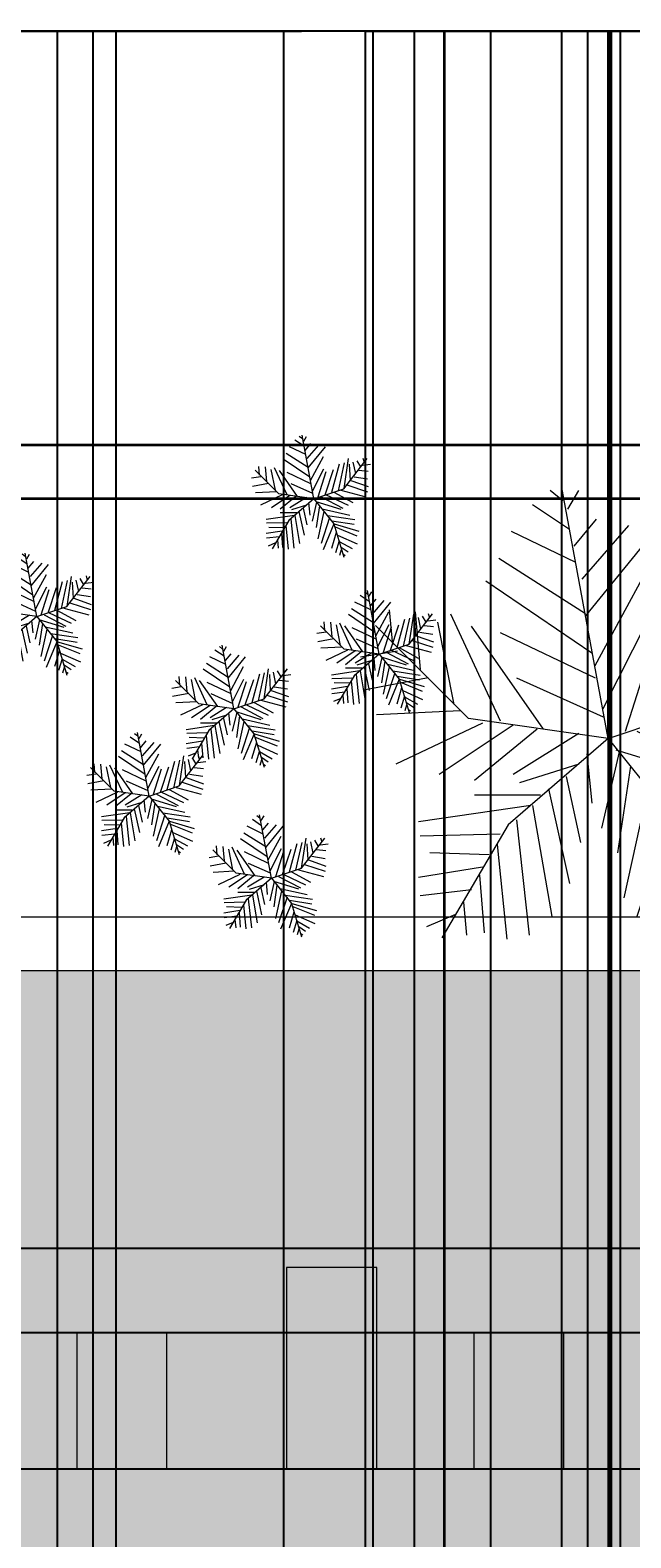
# Model space of a CAD drawing. Units: inches. Extents: x 818 to 1898, y 976 to 2364.
# Tile 95 of 96: x 1612 to 1713, y 2111 to 2364. Entities that reach past the tile are written whole.
import ezdxf

# ---------------------------------------------------------------- set-up
doc = ezdxf.new("R2010")
doc.units = ezdxf.units.IN
doc.header["$LTSCALE"] = 5
doc.header["$MEASUREMENT"] = 0
for name, color, linetype, lineweight in [('A-ANNO-DIMS', 2, 'Continuous', 18), ('C-PROP', 7, 'Continuous', 35), ('L-PAVE', 8, 'Continuous', 18), ('L-PLNT-BEDS', 94, 'Continuous', 18)]:
    doc.layers.add(name, color=color, linetype=linetype, lineweight=lineweight)
for name, color, linetype, lineweight, true_color in [('L-PAVE-PATT', 9, 'Continuous', 9, 0xc7c8ca), ('L-PLNT', 116, 'Continuous', 13, 0x136734), ('L-PLNT-PATT', 114, 'Continuous', 9, 0x139b48)]:
    doc.layers.add(name, color=color, linetype=linetype, lineweight=lineweight, true_color=true_color)
doc.styles.get("Standard").update_dxf_attribs({"font": 'arial.ttf'})
doc.dimstyles.get("Standard").update_dxf_attribs({"dimtxt": 0.18, "dimasz": 0.18, "dimexe": 0.18, "dimexo": 0.0625, "dimgap": 0.09, "dimtad": 0, "dimtih": 1, "dimtoh": 1, "dimdec": 4, "dimzin": 0, "dimdsep": 46, "dimtxsty": 'Standard', "dimcen": 0.09, "dimadec": 0, "dimazin": 0, "dimtfac": 1, "dimtdec": 4, "dimtofl": 0, "dimtmove": 0, "dimatfit": 3, "dimfxl": 1, "dimtolj": 1, "dimtzin": 0, "dimarcsym": 0})

# ---------------------------------------------------------------- blocks, each defined once
blk = doc.blocks.new('SHRUB-ACCENT')
for p, q in [((8.53, 19.84), (7.99, 20.28)), ((10.44, 9.82), (8.47, 20.47)), ((8.74, 19.5), (9.21, 20.28)), ((9.08, 17.24), (6.37, 18.54)), ((8.8, 18.63), (7.25, 19.67)), ((9.01, 17.93), (9.96, 19.06)), ((9.35, 16.54), (11.31, 18.8)), ((9.48, 14.98), (12.39, 18.54)), ((1.35, 13.77), (1.22, 15.24)), ((9.75, 13.42), (5.28, 16.46)), ((9.48, 15.07), (5.82, 17.41)), ((9.89, 12.9), (12.06, 16.89)), ((13.48, 10.9), (14.76, 15.68)), ((14.56, 11.16), (15.58, 15.85)), ((15.49, 11.5), (19.41, 16.55)), ((15.51, 11.51), (16.25, 16.54)), ((16.39, 15.59), (16.53, 12.9)), ((17, 15.94), (17.41, 14.03)), ((17.68, 16.2), (18.29, 15.16)), ((18.62, 15.42), (19.98, 15.59)), ((18.69, 16.63), (18.9, 15.94)), ((1.56, 13.51), (0, 13.25)), ((4.55, 10.66), (0.62, 14.58)), ((2.3, 15.16), (2.51, 12.72)), ((3.25, 14.72), (3.93, 11.25)), ((3.79, 15.07), (5.89, 10.55)), ((7.72, 10.21), (4.67, 14.55)), ((5.89, 14.29), (9.89, 12.38)), ((10.23, 11.07), (12.12, 14.81)), ((11.17, 10.12), (12.53, 14.37)), ((12.33, 10.47), (13.75, 14.72)), ((16.66, 12.9), (19.57, 11.86)), ((17.2, 13.51), (19.44, 13.16)), ((18.02, 14.63), (19.57, 14.46)), ((2.84, 12.38), (0.14, 11.86)), ((4.2, 10.99), (0.68, 10.81)), ((5.15, 10.47), (1.49, 8.73)), ((6.43, 10.38), (3.32, 8.3)), ((10.44, 9.82), (4.55, 10.66)), ((7.45, 10.21), (4.81, 8.04)), ((6.57, 12.38), (10.23, 10.73)), ((10.44, 9.82), (15.49, 11.5)), ((12.53, 10.47), (16.19, 8.73)), ((13.82, 10.9), (17, 9.16)), ((14.97, 11.25), (19.17, 10.12)), ((15.98, 12.12), (19.44, 10.99)), ((10.44, 9.82), (6.23, 6.17)), ((9.21, 10.03), (6.43, 8.3)), ((9.21, 8.73), (6.7, 7.95)), ((7.92, 7.69), (8.8, 3.69)), ((8.67, 8.21), (9.28, 5.43)), ((9.55, 9.16), (9.75, 7.08)), ((10.9, 9.25), (10.16, 6.04)), ((10.44, 9.82), (13.8, 5.61)), ((10.77, 9.34), (14.97, 8.04)), ((11.38, 8.64), (10.84, 5)), ((12.12, 7.69), (11.11, 3.09)), ((11.65, 10.12), (15.31, 8.21)), ((11.85, 8.12), (16.46, 7.08)), ((7.18, 6.99), (2.44, 6.3)), ((5.89, 5.78), (2.51, 5.69)), ((6.23, 6.17), (3.43, 1.4)), ((7.59, 7.43), (4.81, 7.43)), ((5.76, 5.34), (6.16, 1.35)), ((6.57, 6.39), (7.11, 1.52)), ((7.25, 6.99), (8.06, 2.31)), ((13.07, 6.65), (11.65, 2.31)), ((13.82, 5.6), (11.99, 1.26)), ((12.73, 6.99), (17.34, 6.3)), ((13.48, 6.13), (17.2, 5.52)), ((13.8, 5.61), (15.49, 0)), ((13.88, 5.6), (18.02, 4.39)), ((14.02, 5.08), (17.68, 3.61)), ((5.15, 4.39), (2.44, 3.95)), ((4.67, 3.43), (2.51, 3.17)), ((5.42, 4.91), (2.91, 5)), ((4.33, 2.91), (4.47, 1.52)), ((5.01, 4.04), (5.21, 1.61)), ((14.22, 4.13), (13.41, 1.44)), ((14.7, 2.74), (14.09, 0.74)), ((14.43, 3.69), (17.74, 2.22)), ((14.7, 2.65), (16.86, 1.44)), ((4, 2.39), (2.78, 1.87)), ((15.04, 1.26), (14.76, 0.31)), ((15.04, 1.7), (16.19, 0.92)), ((15.44, 0.48), (15.71, 0.31))]:
    blk.add_line(p, q)
blk = doc.blocks.new('PALM-BORDER')
for p, q in [((41.53, 39.05), (33.72, 81.45)), ((33.95, 78.95), (31.8, 80.68)), ((34.76, 77.57), (36.65, 80.68)), ((35.03, 74.11), (28.83, 78.26)), ((36.11, 68.59), (25.33, 73.77)), ((35.84, 71.35), (39.61, 75.84)), ((37.18, 65.82), (45, 74.8)), ((37.72, 59.6), (49.31, 73.77)), ((37.72, 59.95), (23.17, 69.28)), ((39.34, 51.31), (47.96, 67.2)), ((61.61, 45.75), (77.23, 65.83)), ((61.71, 45.79), (64.67, 65.82)), ((74.37, 66.17), (75.18, 63.4)), ((38.8, 53.39), (21.02, 65.48)), ((67.63, 63.4), (69.25, 55.81)), ((70.33, 64.44), (72.75, 60.3)), ((53.62, 43.37), (58.74, 62.37)), ((57.93, 44.41), (61.97, 63.06)), ((65.21, 62.02), (65.75, 51.31)), ((74.1, 61.33), (79.49, 62.02)), ((5.39, 54.77), (4.85, 60.64)), ((9.16, 60.3), (9.97, 50.62)), ((12.93, 58.57), (15.63, 44.75)), ((15.09, 59.95), (23.44, 41.99)), ((40.69, 44.06), (48.23, 58.91)), ((49.04, 41.64), (54.7, 58.57)), ((71.68, 58.22), (77.87, 57.53)), ((18.1, 42.4), (2.48, 58.02)), ((30.72, 40.61), (18.59, 57.88)), ((23.44, 56.84), (39.34, 49.24)), ((44.46, 40.26), (49.85, 57.19)), ((6.2, 53.73), (0, 52.7)), ((68.44, 53.73), (77.33, 52.35)), ((66.29, 51.31), (77.87, 47.17)), ((11.32, 49.24), (0.54, 47.17)), ((26.14, 49.24), (40.69, 42.68)), ((63.59, 48.21), (77.33, 43.71)), ((41.53, 39.05), (61.61, 45.75)), ((16.71, 43.71), (2.69, 43.02)), ((54.97, 43.37), (67.63, 36.46)), ((59.55, 44.75), (76.26, 40.26)), ((20.48, 41.64), (5.93, 34.73)), ((25.6, 41.3), (13.2, 33.01)), ((41.53, 39.05), (18.1, 42.4)), ((29.64, 40.61), (19.13, 31.97)), ((49.85, 41.64), (64.4, 34.73)), ((41.53, 39.05), (24.79, 24.55)), ((36.65, 39.91), (25.6, 33.01)), ((41.53, 39.05), (54.92, 22.32)), ((46.35, 40.26), (60.9, 32.66)), ((37.99, 36.46), (38.8, 28.17)), ((43.38, 36.81), (40.42, 24.02)), ((42.84, 37.15), (59.55, 31.97)), ((36.65, 34.73), (26.68, 31.62)), ((45.27, 34.39), (43.11, 19.88)), ((31.53, 30.59), (35.03, 14.7)), ((34.49, 32.66), (36.92, 21.61)), ((48.23, 30.59), (44.19, 12.28)), ((47.15, 32.32), (65.48, 28.17)), ((30.18, 29.55), (19.13, 29.55)), ((28.56, 27.82), (9.7, 25.06)), ((26.14, 25.41), (28.29, 6.06)), ((28.83, 27.82), (32.07, 9.17)), ((52, 26.44), (46.35, 9.17)), ((50.66, 27.82), (68.98, 25.06)), ((23.44, 22.99), (9.97, 22.64)), ((24.79, 24.55), (13.63, 5.58)), ((53.62, 24.37), (68.44, 21.95)), ((22.9, 21.26), (24.52, 5.37)), ((54.97, 22.3), (47.69, 5.02)), ((54.92, 22.32), (61.61, 0)), ((55.24, 22.3), (71.68, 17.46)), ((21.56, 19.53), (11.59, 19.88)), ((55.78, 20.22), (70.33, 14.35)), ((20.48, 17.46), (9.7, 15.73)), ((19.94, 16.08), (20.75, 6.41)), ((56.59, 16.42), (53.35, 5.72)), ((18.59, 13.66), (9.97, 12.62)), ((57.39, 14.7), (70.6, 8.83)), ((17.24, 11.59), (17.78, 6.06)), ((58.47, 10.9), (56.05, 2.95)), ((58.47, 10.55), (67.09, 5.72)), ((15.9, 9.52), (11.05, 7.44)), ((59.82, 6.75), (64.4, 3.64)), ((59.82, 5.02), (58.74, 1.22)), ((61.44, 1.92), (62.51, 1.22))]:
    blk.add_line(p, q)
blk = doc.blocks.new('*D57')
at = {"layer": 'A-ANNO-DIMS', "color": 0, "lineweight": -2, "ltscale": 5, "transparency": 16777216}
for p, q in [((992.73, 2294.28), (992.73, 2363.87)), ((992.91, 2363.69), (1395.43, 2363.69)), ((1798.54, 2363.69), (1396.01, 2363.69)), ((1798.72, 2294.28), (1798.72, 2363.87))]:
    blk.add_line(p, q, dxfattribs=at)
at = {"layer": 'A-ANNO-DIMS', "color": 0, "ltscale": 5, "transparency": 16777216}
for points in [[(992.91, 2363.72), (992.91, 2363.66), (992.73, 2363.69)], [(1798.54, 2363.72), (1798.54, 2363.66), (1798.72, 2363.69)]]:
    blk.add_solid(points, dxfattribs=at)
at = {"layer": 'Defpoints', "color": 0, "ltscale": 5, "transparency": 16777216}
for p in [(1798.72, 2363.69), (992.73, 2294.22), (1798.72, 2294.22)]:
    blk.add_point(p, dxfattribs=at)
at = {"layer": 'A-ANNO-DIMS', "color": 0, "ltscale": 5, "transparency": 16777216, "insert": (1395.72, 2363.69), "char_height": 0.18, "attachment_point": 5}
blk.add_mtext('\\A1;806', dxfattribs=at)
blk = doc.blocks.new('*D86')
at = {"layer": 'A-ANNO-DIMS', "color": 0, "lineweight": -2, "ltscale": 5, "transparency": 16777216}
for p, q in [((1258.73, 2053.14), (1258.73, 2363.87)), ((1258.91, 2363.69), (1486.43, 2363.69)), ((1714.55, 2363.69), (1487.02, 2363.69)), ((1714.73, 2053.14), (1714.73, 2363.87))]:
    blk.add_line(p, q, dxfattribs=at)
at = {"layer": 'A-ANNO-DIMS', "color": 0, "ltscale": 5, "transparency": 16777216}
for points in [[(1258.91, 2363.72), (1258.91, 2363.66), (1258.73, 2363.69)], [(1714.55, 2363.72), (1714.55, 2363.66), (1714.73, 2363.69)]]:
    blk.add_solid(points, dxfattribs=at)
at = {"layer": 'Defpoints', "color": 0, "ltscale": 5, "transparency": 16777216}
for p in [(1714.73, 2363.69), (1258.73, 2053.08), (1714.73, 2053.08)]:
    blk.add_point(p, dxfattribs=at)
at = {"layer": 'A-ANNO-DIMS', "color": 0, "ltscale": 5, "transparency": 16777216, "insert": (1486.73, 2363.69), "char_height": 0.18, "attachment_point": 5}
blk.add_mtext('\\A1;456', dxfattribs=at)
blk = doc.blocks.new('*D102')
at = {"layer": 'A-ANNO-DIMS', "color": 0, "lineweight": -2, "ltscale": 5, "transparency": 16777216}
for p, q in [((1565.48, 1071.12), (1565.48, 2363.87)), ((1565.66, 2363.69), (1595.63, 2363.69)), ((1626.39, 2363.69), (1596.42, 2363.69)), ((1626.57, 1071.12), (1626.57, 2363.87))]:
    blk.add_line(p, q, dxfattribs=at)
at = {"layer": 'A-ANNO-DIMS', "color": 0, "ltscale": 5, "transparency": 16777216}
for points in [[(1565.66, 2363.72), (1565.66, 2363.66), (1565.48, 2363.69)], [(1626.39, 2363.72), (1626.39, 2363.66), (1626.57, 2363.69)]]:
    blk.add_solid(points, dxfattribs=at)
at = {"layer": 'Defpoints', "color": 0, "ltscale": 5, "transparency": 16777216}
for p in [(1626.57, 2363.69), (1565.48, 1071.06), (1626.57, 1071.06)]:
    blk.add_point(p, dxfattribs=at)
at = {"layer": 'A-ANNO-DIMS', "color": 0, "ltscale": 5, "transparency": 16777216, "insert": (1596.03, 2363.69), "char_height": 0.18, "attachment_point": 5}
blk.add_mtext('\\A1;61.09', dxfattribs=at)
blk = doc.blocks.new('*D103')
at = {"layer": 'A-ANNO-DIMS', "color": 0, "lineweight": -2, "ltscale": 5, "transparency": 16777216}
for p, q in [((1626.57, 1071.12), (1626.57, 2363.87)), ((1626.75, 2363.69), (1657.7, 2363.69)), ((1689.29, 2363.69), (1658.35, 2363.69)), ((1689.47, 1071.12), (1689.47, 2363.87))]:
    blk.add_line(p, q, dxfattribs=at)
at = {"layer": 'A-ANNO-DIMS', "color": 0, "ltscale": 5, "transparency": 16777216}
for points in [[(1626.75, 2363.72), (1626.75, 2363.66), (1626.57, 2363.69)], [(1689.29, 2363.72), (1689.29, 2363.66), (1689.47, 2363.69)]]:
    blk.add_solid(points, dxfattribs=at)
at = {"layer": 'Defpoints', "color": 0, "ltscale": 5, "transparency": 16777216}
for p in [(1689.47, 2363.69), (1626.57, 1071.06), (1689.47, 1071.06)]:
    blk.add_point(p, dxfattribs=at)
at = {"layer": 'A-ANNO-DIMS', "color": 0, "ltscale": 5, "transparency": 16777216, "insert": (1658.02, 2363.69), "char_height": 0.18, "attachment_point": 5}
blk.add_mtext('\\A1;62.9', dxfattribs=at)
blk = doc.blocks.new('*D104')
at = {"layer": 'A-ANNO-DIMS', "color": 0, "lineweight": -2, "ltscale": 5, "transparency": 16777216}
for p, q in [((1689.47, 1071.12), (1689.47, 2363.87)), ((1689.65, 2363.69), (1717.4, 2363.69)), ((1745.9, 2363.69), (1718.15, 2363.69)), ((1746.08, 1071.12), (1746.08, 2363.87))]:
    blk.add_line(p, q, dxfattribs=at)
at = {"layer": 'A-ANNO-DIMS', "color": 0, "ltscale": 5, "transparency": 16777216}
for points in [[(1689.65, 2363.72), (1689.65, 2363.66), (1689.47, 2363.69)], [(1745.9, 2363.72), (1745.9, 2363.66), (1746.08, 2363.69)]]:
    blk.add_solid(points, dxfattribs=at)
at = {"layer": 'Defpoints', "color": 0, "ltscale": 5, "transparency": 16777216}
for p in [(1746.08, 2363.69), (1689.47, 1071.06), (1746.08, 1071.06)]:
    blk.add_point(p, dxfattribs=at)
at = {"layer": 'A-ANNO-DIMS', "color": 0, "ltscale": 5, "transparency": 16777216, "insert": (1717.78, 2363.69), "char_height": 0.18, "attachment_point": 5}
blk.add_mtext('\\A1;56.61', dxfattribs=at)
blk = doc.blocks.new('*D139')
at = {"layer": 'A-ANNO-DIMS', "color": 0, "lineweight": -2, "ltscale": 5, "transparency": 16777216}
for p, q in [((1550.87, 2253.22), (1550.87, 2363.87)), ((1551.05, 2363.69), (1629.62, 2363.69)), ((1708.97, 2363.69), (1630.39, 2363.69)), ((1709.15, 2245.03), (1709.15, 2363.87))]:
    blk.add_line(p, q, dxfattribs=at)
at = {"layer": 'A-ANNO-DIMS', "color": 0, "ltscale": 5, "transparency": 16777216}
for points in [[(1551.05, 2363.72), (1551.05, 2363.66), (1550.87, 2363.69)], [(1708.97, 2363.72), (1708.97, 2363.66), (1709.15, 2363.69)]]:
    blk.add_solid(points, dxfattribs=at)
at = {"layer": 'Defpoints', "color": 0, "ltscale": 5, "transparency": 16777216}
for p in [(1709.15, 2363.69), (1550.87, 2253.16), (1709.15, 2244.97)]:
    blk.add_point(p, dxfattribs=at)
at = {"layer": 'A-ANNO-DIMS', "color": 0, "ltscale": 5, "transparency": 16777216, "insert": (1630.01, 2363.69), "char_height": 0.18, "attachment_point": 5}
blk.add_mtext('\\A1;158.3', dxfattribs=at)
blk = doc.blocks.new('*D147')
at = {"layer": 'A-ANNO-DIMS', "color": 0, "lineweight": -2, "ltscale": 5, "transparency": 16777216}
for p, q in [((1212.58, 2145.25), (1897.92, 2145.25)), ((1897.74, 2145.07), (1897.74, 2133.99)), ((1897.74, 2122.56), (1897.74, 2133.63)), ((1212.58, 2122.38), (1897.92, 2122.38))]:
    blk.add_line(p, q, dxfattribs=at)
at = {"layer": 'A-ANNO-DIMS', "color": 0, "ltscale": 5, "transparency": 16777216}
for points in [[(1897.71, 2145.07), (1897.77, 2145.07), (1897.74, 2145.25)], [(1897.71, 2122.56), (1897.77, 2122.56), (1897.74, 2122.38)]]:
    blk.add_solid(points, dxfattribs=at)
at = {"layer": 'Defpoints', "color": 0, "ltscale": 5, "transparency": 16777216}
for p in [(1212.52, 2145.25), (1897.74, 2145.25), (1212.52, 2122.38)]:
    blk.add_point(p, dxfattribs=at)
at = {"layer": 'A-ANNO-DIMS', "color": 0, "ltscale": 5, "transparency": 16777216, "insert": (1897.74, 2133.81), "char_height": 0.18, "attachment_point": 5}
blk.add_mtext('\\A1;22.87', dxfattribs=at)
blk = doc.blocks.new('*D148')
at = {"layer": 'A-ANNO-DIMS', "color": 0, "lineweight": -2, "ltscale": 5, "transparency": 16777216}
for p, q in [((1232.67, 2159.43), (1897.92, 2159.43)), ((1897.74, 2159.25), (1897.74, 2141.09)), ((1897.74, 2122.56), (1897.74, 2140.72)), ((1232.67, 2122.38), (1897.92, 2122.38))]:
    blk.add_line(p, q, dxfattribs=at)
at = {"layer": 'A-ANNO-DIMS', "color": 0, "ltscale": 5, "transparency": 16777216}
for points in [[(1897.71, 2159.25), (1897.77, 2159.25), (1897.74, 2159.43)], [(1897.71, 2122.56), (1897.77, 2122.56), (1897.74, 2122.38)]]:
    blk.add_solid(points, dxfattribs=at)
at = {"layer": 'Defpoints', "color": 0, "ltscale": 5, "transparency": 16777216}
for p in [(1232.61, 2159.43), (1897.74, 2159.43), (1232.61, 2122.38)]:
    blk.add_point(p, dxfattribs=at)
at = {"layer": 'A-ANNO-DIMS', "color": 0, "ltscale": 5, "transparency": 16777216, "insert": (1897.74, 2140.9), "char_height": 0.18, "attachment_point": 5}
blk.add_mtext('\\A1;37.05', dxfattribs=at)
blk = doc.blocks.new('*D154')
at = {"layer": 'A-ANNO-DIMS', "color": 0, "lineweight": -2, "ltscale": 5, "transparency": 16777216}
for p, q in [((1701.37, 1290.14), (1701.37, 2363.87)), ((1701.55, 2363.69), (1705.22, 2363.69)), ((1709.19, 2363.69), (1705.52, 2363.69)), ((1709.37, 1298.14), (1709.37, 2363.87))]:
    blk.add_line(p, q, dxfattribs=at)
at = {"layer": 'A-ANNO-DIMS', "color": 0, "ltscale": 5, "transparency": 16777216}
for points in [[(1701.55, 2363.72), (1701.55, 2363.66), (1701.37, 2363.69)], [(1709.19, 2363.72), (1709.19, 2363.66), (1709.37, 2363.69)]]:
    blk.add_solid(points, dxfattribs=at)
at = {"layer": 'Defpoints', "color": 0, "ltscale": 5, "transparency": 16777216}
for p in [(1709.37, 2363.69), (1709.37, 1298.08), (1701.37, 1290.08)]:
    blk.add_point(p, dxfattribs=at)
at = {"layer": 'A-ANNO-DIMS', "color": 0, "ltscale": 5, "transparency": 16777216, "insert": (1705.37, 2363.69), "char_height": 0.18, "attachment_point": 5}
blk.add_mtext('\\A1;8', dxfattribs=at)
blk = doc.blocks.new('*D173')
at = {"layer": 'A-ANNO-DIMS', "color": 0, "lineweight": -2, "ltscale": 5, "transparency": 16777216}
for p, q in [((1622.73, 1463.14), (1622.73, 2363.87)), ((1622.91, 2363.69), (1638.51, 2363.69)), ((1654.55, 2363.69), (1638.94, 2363.69)), ((1654.73, 1463.14), (1654.73, 2363.87))]:
    blk.add_line(p, q, dxfattribs=at)
at = {"layer": 'A-ANNO-DIMS', "color": 0, "ltscale": 5, "transparency": 16777216}
for points in [[(1622.91, 2363.72), (1622.91, 2363.66), (1622.73, 2363.69)], [(1654.55, 2363.72), (1654.55, 2363.66), (1654.73, 2363.69)]]:
    blk.add_solid(points, dxfattribs=at)
at = {"layer": 'Defpoints', "color": 0, "ltscale": 5, "transparency": 16777216}
for p in [(1654.73, 2363.69), (1622.73, 1463.08), (1654.73, 1463.08)]:
    blk.add_point(p, dxfattribs=at)
at = {"layer": 'A-ANNO-DIMS', "color": 0, "ltscale": 5, "transparency": 16777216, "insert": (1638.73, 2363.69), "char_height": 0.18, "attachment_point": 5}
blk.add_mtext('\\A1;32', dxfattribs=at)
blk = doc.blocks.new('*D174')
at = {"layer": 'A-ANNO-DIMS', "color": 0, "lineweight": -2, "ltscale": 5, "transparency": 16777216}
for p, q in [((1616.73, 1416.75), (1616.73, 2363.87)), ((1616.91, 2363.69), (1619.58, 2363.69)), ((1622.55, 2363.69), (1619.87, 2363.69)), ((1622.73, 1416.75), (1622.73, 2363.87))]:
    blk.add_line(p, q, dxfattribs=at)
at = {"layer": 'A-ANNO-DIMS', "color": 0, "ltscale": 5, "transparency": 16777216}
for points in [[(1616.91, 2363.72), (1616.91, 2363.66), (1616.73, 2363.69)], [(1622.55, 2363.72), (1622.55, 2363.66), (1622.73, 2363.69)]]:
    blk.add_solid(points, dxfattribs=at)
at = {"layer": 'Defpoints', "color": 0, "ltscale": 5, "transparency": 16777216}
for p in [(1622.73, 2363.69), (1616.73, 1416.69), (1622.73, 1416.69)]:
    blk.add_point(p, dxfattribs=at)
at = {"layer": 'A-ANNO-DIMS', "color": 0, "ltscale": 5, "transparency": 16777216, "insert": (1619.73, 2363.69), "char_height": 0.18, "attachment_point": 5}
blk.add_mtext('\\A1;6', dxfattribs=at)
blk = doc.blocks.new('*D175')
at = {"layer": 'A-ANNO-DIMS', "color": 0, "lineweight": -2, "ltscale": 5, "transparency": 16777216}
for p, q in [((1559.73, 1647.64), (1559.73, 2363.87)), ((1559.91, 2363.69), (1614.45, 2363.69)), ((1669.55, 2363.69), (1615.01, 2363.69)), ((1669.73, 1647.64), (1669.73, 2363.87))]:
    blk.add_line(p, q, dxfattribs=at)
at = {"layer": 'A-ANNO-DIMS', "color": 0, "ltscale": 5, "transparency": 16777216}
for points in [[(1559.91, 2363.72), (1559.91, 2363.66), (1559.73, 2363.69)], [(1669.55, 2363.72), (1669.55, 2363.66), (1669.73, 2363.69)]]:
    blk.add_solid(points, dxfattribs=at)
at = {"layer": 'Defpoints', "color": 0, "ltscale": 5, "transparency": 16777216}
for p in [(1669.73, 2363.69), (1559.73, 1647.58), (1669.73, 1647.58)]:
    blk.add_point(p, dxfattribs=at)
at = {"layer": 'A-ANNO-DIMS', "color": 0, "ltscale": 5, "transparency": 16777216, "insert": (1614.73, 2363.69), "char_height": 0.18, "attachment_point": 5}
blk.add_mtext('\\A1;110', dxfattribs=at)
blk = doc.blocks.new('*D195')
at = {"layer": 'A-ANNO-DIMS', "color": 0, "lineweight": -2, "ltscale": 5, "transparency": 16777216}
for p, q in [((1681.73, 1379.14), (1681.73, 2363.87)), ((1681.91, 2363.69), (1693.51, 2363.69)), ((1705.55, 2363.69), (1693.95, 2363.69)), ((1705.73, 1355.14), (1705.73, 2363.87))]:
    blk.add_line(p, q, dxfattribs=at)
at = {"layer": 'A-ANNO-DIMS', "color": 0, "ltscale": 5, "transparency": 16777216}
for points in [[(1681.91, 2363.72), (1681.91, 2363.66), (1681.73, 2363.69)], [(1705.55, 2363.72), (1705.55, 2363.66), (1705.73, 2363.69)]]:
    blk.add_solid(points, dxfattribs=at)
at = {"layer": 'Defpoints', "color": 0, "ltscale": 5, "transparency": 16777216}
for p in [(1705.73, 2363.69), (1681.73, 1379.08), (1705.73, 1355.08)]:
    blk.add_point(p, dxfattribs=at)
at = {"layer": 'A-ANNO-DIMS', "color": 0, "ltscale": 5, "transparency": 16777216, "insert": (1693.73, 2363.69), "char_height": 0.18, "attachment_point": 5}
blk.add_mtext('\\A1;24', dxfattribs=at)
blk = doc.blocks.new('*D203')
at = {"layer": 'A-ANNO-DIMS', "color": 0, "lineweight": -2, "ltscale": 5, "transparency": 16777216}
for p, q in [((1599.73, 1876.14), (1599.73, 2363.87)), ((1599.91, 2363.69), (1652.44, 2363.69)), ((1705.55, 2363.69), (1653.01, 2363.69)), ((1705.73, 1876.14), (1705.73, 2363.87))]:
    blk.add_line(p, q, dxfattribs=at)
at = {"layer": 'A-ANNO-DIMS', "color": 0, "ltscale": 5, "transparency": 16777216}
for points in [[(1599.91, 2363.72), (1599.91, 2363.66), (1599.73, 2363.69)], [(1705.55, 2363.72), (1705.55, 2363.66), (1705.73, 2363.69)]]:
    blk.add_solid(points, dxfattribs=at)
at = {"layer": 'Defpoints', "color": 0, "ltscale": 5, "transparency": 16777216}
for p in [(1705.73, 2363.69), (1599.73, 1876.08), (1705.73, 1876.08)]:
    blk.add_point(p, dxfattribs=at)
at = {"layer": 'A-ANNO-DIMS', "color": 0, "ltscale": 5, "transparency": 16777216, "insert": (1652.73, 2363.69), "char_height": 0.18, "attachment_point": 5}
blk.add_mtext('\\A1;106', dxfattribs=at)
blk = doc.blocks.new('*D205')
at = {"layer": 'A-ANNO-DIMS', "color": 0, "lineweight": -2, "ltscale": 5, "transparency": 16777216}
for p, q in [((1590.73, 2044.14), (1590.73, 2363.87)), ((1590.91, 2363.69), (1652.45, 2363.69)), ((1714.55, 2363.69), (1653.01, 2363.69)), ((1714.73, 2053.14), (1714.73, 2363.87))]:
    blk.add_line(p, q, dxfattribs=at)
at = {"layer": 'A-ANNO-DIMS', "color": 0, "ltscale": 5, "transparency": 16777216}
for points in [[(1590.91, 2363.72), (1590.91, 2363.66), (1590.73, 2363.69)], [(1714.55, 2363.72), (1714.55, 2363.66), (1714.73, 2363.69)]]:
    blk.add_solid(points, dxfattribs=at)
at = {"layer": 'Defpoints', "color": 0, "ltscale": 5, "transparency": 16777216}
for p in [(1714.73, 2363.69), (1714.73, 2053.08), (1590.73, 2044.08)]:
    blk.add_point(p, dxfattribs=at)
at = {"layer": 'A-ANNO-DIMS', "color": 0, "ltscale": 5, "transparency": 16777216, "insert": (1652.73, 2363.69), "char_height": 0.18, "attachment_point": 5}
blk.add_mtext('\\A1;124', dxfattribs=at)
blk = doc.blocks.new('*D213')
at = {"layer": 'A-ANNO-DIMS', "color": 0, "lineweight": -2, "ltscale": 5, "transparency": 16777216}
for p, q in [((1709.23, 1962.1), (1709.23, 2363.87)), ((1709.41, 2363.69), (1710.08, 2363.69)), ((1711.05, 2363.69), (1710.37, 2363.69)), ((1711.23, 1962.1), (1711.23, 2363.87))]:
    blk.add_line(p, q, dxfattribs=at)
at = {"layer": 'A-ANNO-DIMS', "color": 0, "ltscale": 5, "transparency": 16777216}
for points in [[(1709.41, 2363.72), (1709.41, 2363.66), (1709.23, 2363.69)], [(1711.05, 2363.72), (1711.05, 2363.66), (1711.23, 2363.69)]]:
    blk.add_solid(points, dxfattribs=at)
at = {"layer": 'Defpoints', "color": 0, "ltscale": 5, "transparency": 16777216}
for p in [(1711.23, 2363.69), (1709.23, 1962.03), (1711.23, 1962.03)]:
    blk.add_point(p, dxfattribs=at)
at = {"layer": 'A-ANNO-DIMS', "color": 0, "ltscale": 5, "transparency": 16777216, "insert": (1710.23, 2363.69), "char_height": 0.18, "attachment_point": 5}
blk.add_mtext('\\A1;2', dxfattribs=at)
blk = doc.blocks.new('*D230')
at = {"layer": 'A-ANNO-DIMS', "color": 0, "lineweight": -2, "ltscale": 5, "transparency": 16777216}
for p, q in [((1668.44, 2044.14), (1668.44, 2363.87)), ((1668.62, 2363.69), (1686.69, 2363.69)), ((1705.55, 2363.69), (1687.48, 2363.69)), ((1705.73, 2044.14), (1705.73, 2363.87))]:
    blk.add_line(p, q, dxfattribs=at)
at = {"layer": 'A-ANNO-DIMS', "color": 0, "ltscale": 5, "transparency": 16777216}
for points in [[(1668.62, 2363.72), (1668.62, 2363.66), (1668.44, 2363.69)], [(1705.55, 2363.72), (1705.55, 2363.66), (1705.73, 2363.69)]]:
    blk.add_solid(points, dxfattribs=at)
at = {"layer": 'Defpoints', "color": 0, "ltscale": 5, "transparency": 16777216}
for p in [(1705.73, 2363.69), (1668.44, 2044.08), (1705.73, 2044.08)]:
    blk.add_point(p, dxfattribs=at)
at = {"layer": 'A-ANNO-DIMS', "color": 0, "ltscale": 5, "transparency": 16777216, "insert": (1687.08, 2363.69), "char_height": 0.18, "attachment_point": 5}
blk.add_mtext('\\A1;37.28', dxfattribs=at)
blk = doc.blocks.new('*D259')
at = {"layer": 'A-ANNO-DIMS', "color": 0, "lineweight": -2, "ltscale": 5, "transparency": 16777216}
for p, q in [((1681.64, 2053.14), (1681.64, 2363.87)), ((1681.82, 2363.69), (1695.29, 2363.69)), ((1709.55, 2363.69), (1696.08, 2363.69)), ((1709.73, 2077.25), (1709.73, 2363.87))]:
    blk.add_line(p, q, dxfattribs=at)
at = {"layer": 'A-ANNO-DIMS', "color": 0, "ltscale": 5, "transparency": 16777216}
for points in [[(1681.82, 2363.72), (1681.82, 2363.66), (1681.64, 2363.69)], [(1709.55, 2363.72), (1709.55, 2363.66), (1709.73, 2363.69)]]:
    blk.add_solid(points, dxfattribs=at)
at = {"layer": 'Defpoints', "color": 0, "ltscale": 5, "transparency": 16777216}
for p in [(1709.73, 2363.69), (1709.73, 2077.19), (1681.64, 2053.08)]:
    blk.add_point(p, dxfattribs=at)
at = {"layer": 'A-ANNO-DIMS', "color": 0, "ltscale": 5, "transparency": 16777216, "insert": (1695.68, 2363.69), "char_height": 0.18, "attachment_point": 5}
blk.add_mtext('\\A1;28.08', dxfattribs=at)
blk = doc.blocks.new('*D261')
at = {"layer": 'A-ANNO-DIMS', "color": 0, "lineweight": -2, "ltscale": 5, "transparency": 16777216}
for p, q in [((1676.64, 2081.25), (1676.64, 2363.87)), ((1676.82, 2363.69), (1678.99, 2363.69)), ((1681.46, 2363.69), (1679.29, 2363.69)), ((1681.64, 2077.25), (1681.64, 2363.87))]:
    blk.add_line(p, q, dxfattribs=at)
at = {"layer": 'A-ANNO-DIMS', "color": 0, "ltscale": 5, "transparency": 16777216}
for points in [[(1676.82, 2363.72), (1676.82, 2363.66), (1676.64, 2363.69)], [(1681.46, 2363.72), (1681.46, 2363.66), (1681.64, 2363.69)]]:
    blk.add_solid(points, dxfattribs=at)
at = {"layer": 'Defpoints', "color": 0, "ltscale": 5, "transparency": 16777216}
for p in [(1681.64, 2363.69), (1676.64, 2081.19), (1681.64, 2077.19)]:
    blk.add_point(p, dxfattribs=at)
at = {"layer": 'A-ANNO-DIMS', "color": 0, "ltscale": 5, "transparency": 16777216, "insert": (1679.14, 2363.69), "char_height": 0.18, "attachment_point": 5}
blk.add_mtext('\\A1;5', dxfattribs=at)

msp = doc.modelspace()

# ---------------------------------------------------------------- hatches: boundary and pattern name
at = {"layer": 'L-PAVE-PATT', "ltscale": 5}
h = msp.add_hatch(color=256, dxfattribs=at)
h.dxf.hatch_style = 1
h.paths.add_polyline_path([(1212.5206, 2145.2461), (1197.3925, 2145.2461), (1197.3925, 2122.3767), (1212.5206, 2122.3767)])
h.paths.add_polyline_path([(1247.7373, 2159.4296), (1232.6091, 2159.4296), (1232.6091, 2122.3767), (1247.7373, 2122.3767)])
h.paths.add_polyline_path([(1282.9539, 2145.2461), (1267.8258, 2145.2461), (1267.8258, 2122.3767), (1282.9539, 2122.3767)])
h.paths.add_polyline_path([(1318.1705, 2145.2461), (1303.0424, 2145.2461), (1303.0424, 2122.3767), (1318.1705, 2122.3767)])
h.paths.add_polyline_path([(1353.3871, 2155.7839), (1338.259, 2155.7839), (1338.259, 2122.3767), (1353.3871, 2122.3767)])
h.paths.add_polyline_path([(1388.6037, 2145.2461), (1373.4756, 2145.2461), (1373.4756, 2122.3767), (1388.6037, 2122.3767)])
h.paths.add_polyline_path([(1423.8203, 2145.2461), (1408.6922, 2145.2461), (1408.6922, 2122.3767), (1423.8203, 2122.3767)])
h.paths.add_polyline_path([(1459.037, 2158.4222), (1443.9089, 2158.4222), (1443.9089, 2122.3767), (1459.037, 2122.3767)])
h.paths.add_polyline_path([(1494.2536, 2145.2461), (1479.1255, 2145.2461), (1479.1255, 2122.3767), (1494.2536, 2122.3767)])
h.paths.add_polyline_path([(1529.4702, 2145.2461), (1514.3421, 2145.2461), (1514.3421, 2122.3767), (1529.4702, 2122.3767)])
h.paths.add_polyline_path([(1564.6868, 2156.9246), (1549.5587, 2156.9246), (1549.5587, 2122.3767), (1564.6868, 2122.3767)])
h.paths.add_polyline_path([(1599.9034, 2145.2461), (1584.7753, 2145.2461), (1584.7753, 2122.3767), (1599.9034, 2122.3767)])
h.paths.add_polyline_path([(1635.1201, 2145.2461), (1619.9919, 2145.2461), (1619.9919, 2122.3767), (1635.1201, 2122.3767)])
h.paths.add_polyline_path([(1670.3367, 2156.1761), (1655.2086, 2156.1761), (1655.2086, 2122.3767), (1670.3367, 2122.3767)])
h.paths.add_polyline_path([(1701.7273, 2145.2461), (1686.5992, 2145.2461), (1686.5992, 2122.3767), (1701.7273, 2122.3767)])
h.paths.add_polyline_path([(1730.8897, 2145.2461), (1715.7616, 2145.2461), (1715.7616, 2122.3767), (1730.8897, 2122.3767)])
h.paths.add_polyline_path([(1776.3312, 2145.2461), (1753.1652, 2145.2461), (1753.1652, 2115.6891), (1776.3312, 2115.6891)])
at = {"layer": 'L-PLNT-PATT', "ltscale": 5}
h = msp.add_hatch(color=256, dxfattribs=at)
h.dxf.hatch_style = 1
h.paths.add_polyline_path([(1789.7173, 2205.9709), (1083.7252, 2205.9709), (1083.7252, 2083.2623), (1218.1114, 2083.2623), (1218.1114, 2053.0782), (1390.6356, 2053.0782), (1390.6356, 2081.1881), (1399.6356, 2081.1881), (1413.02, 2081.1881), (1422.02, 2081.1881), (1422.02, 2053.0782), (1676.6446, 2053.0782), (1676.6446, 2081.1881), (1714.7251, 2081.1881), (1714.7251, 2081.6235), (1789.7173, 2081.6235)])
h.paths.add_polyline_path([(1388.6037, 2145.2461), (1388.6037, 2122.3767), (1373.4756, 2122.3767), (1373.4756, 2145.2461)], flags=16)
h.paths.add_polyline_path([(1408.6922, 2145.2461), (1423.8203, 2145.2461), (1423.8203, 2122.3767), (1408.6922, 2122.3767)], flags=16)
h.paths.add_polyline_path([(1353.3871, 2155.7839), (1353.3871, 2122.3767), (1338.259, 2122.3767), (1338.259, 2155.7839)], flags=16)
h.paths.add_polyline_path([(1443.9089, 2158.4222), (1459.037, 2158.4222), (1459.037, 2122.3767), (1443.9089, 2122.3767)], flags=16)
h.paths.add_polyline_path([(1318.1705, 2145.2461), (1318.1705, 2122.3767), (1303.0424, 2122.3767), (1303.0424, 2145.2461)], flags=16)
h.paths.add_polyline_path([(1479.1255, 2145.2461), (1494.2536, 2145.2461), (1494.2536, 2122.3767), (1479.1255, 2122.3767)], flags=16)
h.paths.add_polyline_path([(1282.9539, 2145.2461), (1282.9539, 2122.3767), (1267.8258, 2122.3767), (1267.8258, 2145.2461)], flags=16)
h.paths.add_polyline_path([(1514.3421, 2145.2461), (1529.4702, 2145.2461), (1529.4702, 2122.3767), (1514.3421, 2122.3767)], flags=16)
h.paths.add_polyline_path([(1247.7373, 2159.4296), (1247.7373, 2122.3767), (1232.6091, 2122.3767), (1232.6091, 2159.4296)], flags=16)
h.paths.add_polyline_path([(1549.5587, 2156.9246), (1564.6868, 2156.9246), (1564.6868, 2122.3767), (1549.5587, 2122.3767)], flags=16)
h.paths.add_polyline_path([(1212.5206, 2145.2461), (1212.5206, 2122.3767), (1197.3925, 2122.3767), (1197.3925, 2145.2461)], flags=16)
h.paths.add_polyline_path([(1584.7753, 2145.2461), (1599.9034, 2145.2461), (1599.9034, 2122.3767), (1584.7753, 2122.3767)], flags=16)
h.paths.add_polyline_path([(1185.1073, 2104.7786), (1190.6407, 2104.7786), (1185.1073, 2098.2505), (1179.5738, 2104.7786)], flags=16)
h.paths.add_polyline_path([(1619.9919, 2145.2461), (1635.1201, 2145.2461), (1635.1201, 2122.3767), (1619.9919, 2122.3767)], flags=16)
h.paths.add_polyline_path([(1655.2086, 2156.1761), (1670.3367, 2156.1761), (1670.3367, 2122.3767), (1655.2086, 2122.3767)], flags=16)
h.paths.add_polyline_path([(1686.5992, 2145.2461), (1701.7273, 2145.2461), (1701.7273, 2122.3767), (1686.5992, 2122.3767)], flags=16)
h.paths.add_polyline_path([(1715.7616, 2145.2461), (1730.8897, 2145.2461), (1730.8897, 2122.3767), (1715.7616, 2122.3767)], flags=16)
h.paths.add_polyline_path([(1753.1652, 2145.2461), (1776.3312, 2145.2461), (1776.3312, 2115.6891), (1753.1652, 2115.6891)], flags=16)
h.paths.add_polyline_path([(1191.4331, 2146.5159), (1176.7891, 2146.5159), (1176.7891, 2134.1516), (1191.4331, 2134.1516)], flags=24)

# ---------------------------------------------------------------- linework, layer by layer
at = {"layer": 'C-PROP', "ltscale": 5}
for p, q in [((1798.7173, 2294.2171), (992.7251, 2294.2171)), ((1789.7173, 2285.2171), (1001.7252, 2285.2171))]:
    msp.add_line(p, q, dxfattribs=at)
at = {"layer": 'L-PAVE', "ltscale": 5}
for points in [[(1670.3367, 2156.1761), (1655.2086, 2156.1761), (1655.2086, 2122.3767), (1670.3367, 2122.3767)], [(1635.1201, 2145.2461), (1619.9919, 2145.2461), (1619.9919, 2122.3767), (1635.1201, 2122.3767)], [(1701.7273, 2145.2461), (1686.5992, 2145.2461), (1686.5992, 2122.3767), (1701.7273, 2122.3767)]]:
    msp.add_lwpolyline(points, close=True, dxfattribs=at)
at = {"layer": 'L-PLNT-BEDS', "ltscale": 5}
for p, q in [((1789.7173, 2214.9709), (1071.7252, 2214.9709)), ((1789.7173, 2205.9709), (1083.7252, 2205.9709))]:
    msp.add_line(p, q, dxfattribs=at)

# ---------------------------------------------------------------- block references
at = {"layer": 'L-PLNT'}
for name, p in [('SHRUB-ACCENT', (1649.3266, 2275.4016)), ('PALM-BORDER', (1667.6244, 2205.9177)), ('SHRUB-ACCENT', (1602.8454, 2255.617)), ('SHRUB-ACCENT', (1660.2854, 2249.3161)), ('SHRUB-ACCENT', (1635.9266, 2240.1359)), ('SHRUB-ACCENT', (1621.6892, 2225.4917)), ('SHRUB-ACCENT', (1642.2079, 2211.6843))]:
    msp.add_blockref(name, p, dxfattribs=at)

# ---------------------------------------------------------------- dimensions: what is measured, and where the dimension line sits
at = {"layer": 'A-ANNO-DIMS', "ltscale": 5}
for base, p1, p2, override, picture, middle in [((1798.7173, 2363.6929), (992.7251, 2294.2171), (1798.7173, 2294.2171), {"dimdec": 0, "dimlfac": 1, "dimrnd": 0, "dimzin": 0, "dimdsep": 46, "dimlunit": 2}, '*D57', (1395.7212, 2363.6929)), ((1714.7251, 2363.6929), (1258.7251, 2053.0782), (1714.7251, 2053.0782), {"dimdec": 0, "dimlfac": 1, "dimrnd": 0, "dimzin": 0, "dimdsep": 46, "dimlunit": 2}, '*D86', (1486.7251, 2363.6929)), ((1709.1522, 2363.6929), (1550.8651, 2253.1602), (1709.1522, 2244.9688), {"dimdec": 1, "dimlfac": 1, "dimrnd": 0, "dimzin": 0, "dimdsep": 46, "dimlunit": 2}, '*D139', (1630.0087, 2363.6929)), ((1669.7251, 2363.6929), (1559.7251, 1647.5782), (1669.7251, 1647.5782), {"dimdec": 0, "dimlfac": 1, "dimrnd": 0, "dimzin": 0, "dimdsep": 46, "dimlunit": 2}, '*D175', (1614.7251, 2363.6929)), ((1626.5748, 2363.6929), (1565.4835, 1071.0552), (1626.5748, 1071.0552), {"dimdec": 2, "dimlfac": 1, "dimrnd": 0, "dimzin": 0, "dimdsep": 46, "dimlunit": 2}, '*D102', (1596.0291, 2363.6929)), ((1714.7251, 2363.6929), (1590.7251, 2044.0782), (1714.7251, 2053.0782), {"dimdec": 0, "dimlfac": 1, "dimrnd": 0, "dimzin": 0, "dimdsep": 46, "dimlunit": 2}, '*D205', (1652.7251, 2363.6929)), ((1705.7251, 2363.6929), (1599.7251, 1876.0782), (1705.7251, 1876.0782), {"dimdec": 0, "dimlfac": 1, "dimrnd": 0, "dimzin": 0, "dimdsep": 46, "dimlunit": 2}, '*D203', (1652.7251, 2363.6929)), ((1622.7251, 2363.6929), (1616.7251, 1416.6857), (1622.7251, 1416.6857), {"dimdec": 0, "dimlfac": 1, "dimrnd": 0, "dimzin": 0, "dimdsep": 46, "dimlunit": 2}, '*D174', (1619.7251, 2363.6929)), ((1654.7251, 2363.6929), (1622.7251, 1463.0782), (1654.7251, 1463.0782), {"dimdec": 0, "dimlfac": 1, "dimrnd": 0, "dimzin": 0, "dimdsep": 46, "dimlunit": 2}, '*D173', (1638.7251, 2363.6929)), ((1689.4714, 2363.6929), (1626.5748, 1071.0552), (1689.4714, 1071.0552), {"dimdec": 1, "dimlfac": 1, "dimrnd": 0, "dimzin": 0, "dimdsep": 46, "dimlunit": 2}, '*D103', (1658.0231, 2363.6929)), ((1705.7251, 2363.6929), (1668.4429, 2044.0782), (1705.7251, 2044.0782), {"dimdec": 2, "dimlfac": 1, "dimrnd": 0, "dimzin": 0, "dimdsep": 46, "dimlunit": 2}, '*D230', (1687.084, 2363.6929)), ((1681.6446, 2363.6929), (1676.6446, 2081.1881), (1681.6446, 2077.1881), {"dimdec": 0, "dimlfac": 1, "dimrnd": 0, "dimzin": 0, "dimdsep": 46, "dimlunit": 2}, '*D261', (1679.1446, 2363.6929)), ((1709.7251, 2363.6929), (1681.6446, 2053.0782), (1709.7251, 2077.1881), {"dimdec": 2, "dimlfac": 1, "dimrnd": 0, "dimzin": 0, "dimdsep": 46, "dimlunit": 2}, '*D259', (1695.6849, 2363.6929)), ((1705.7251, 2363.6929), (1681.7251, 1379.0782), (1705.7251, 1355.0782), {"dimdec": 0, "dimlfac": 1, "dimrnd": 0, "dimzin": 0, "dimdsep": 46, "dimlunit": 2}, '*D195', (1693.7251, 2363.6929)), ((1746.0831, 2363.6929), (1689.4714, 1071.0552), (1746.0831, 1071.0552), {"dimdec": 2, "dimlfac": 1, "dimrnd": 0, "dimzin": 0, "dimdsep": 46, "dimlunit": 2}, '*D104', (1717.7772, 2363.6929)), ((1709.3688, 2363.6929), (1701.3688, 1290.0782), (1709.3688, 1298.0782), {"dimdec": 0, "dimlfac": 1, "dimrnd": 0, "dimzin": 0, "dimdsep": 46, "dimlunit": 2}, '*D154', (1705.3688, 2363.6929)), ((1711.2251, 2363.6929), (1709.2251, 1962.0338), (1711.2251, 1962.0338), {"dimdec": 0, "dimlfac": 1, "dimrnd": 0, "dimzin": 0, "dimdsep": 46, "dimlunit": 2}, '*D213', (1710.2251, 2363.6929))]:
    dim = msp.add_linear_dim(base=base, p1=p1, p2=p2, dimstyle='Standard', override=override, dxfattribs=at)
    dim.commit()
    dim.dimension.update_dxf_attribs({"geometry": picture, "text_midpoint": middle})
for base, p1, p2, picture, middle in [((1897.736, 2159.4296), (1232.6091, 2122.3767), (1232.6091, 2159.4296), '*D148', (1897.736, 2140.9032)), ((1897.736, 2145.2461), (1212.5206, 2122.3767), (1212.5206, 2145.2461), '*D147', (1897.736, 2133.8114))]:
    dim = msp.add_linear_dim(base=base, p1=p1, p2=p2, angle=90, dimstyle='Standard', override={"dimdec": 2, "dimlfac": 1, "dimrnd": 0, "dimzin": 0, "dimdsep": 46, "dimlunit": 2}, dxfattribs=at)
    dim.commit()
    dim.dimension.update_dxf_attribs({"geometry": picture, "text_midpoint": middle})

doc.saveas('drawing.dxf')
